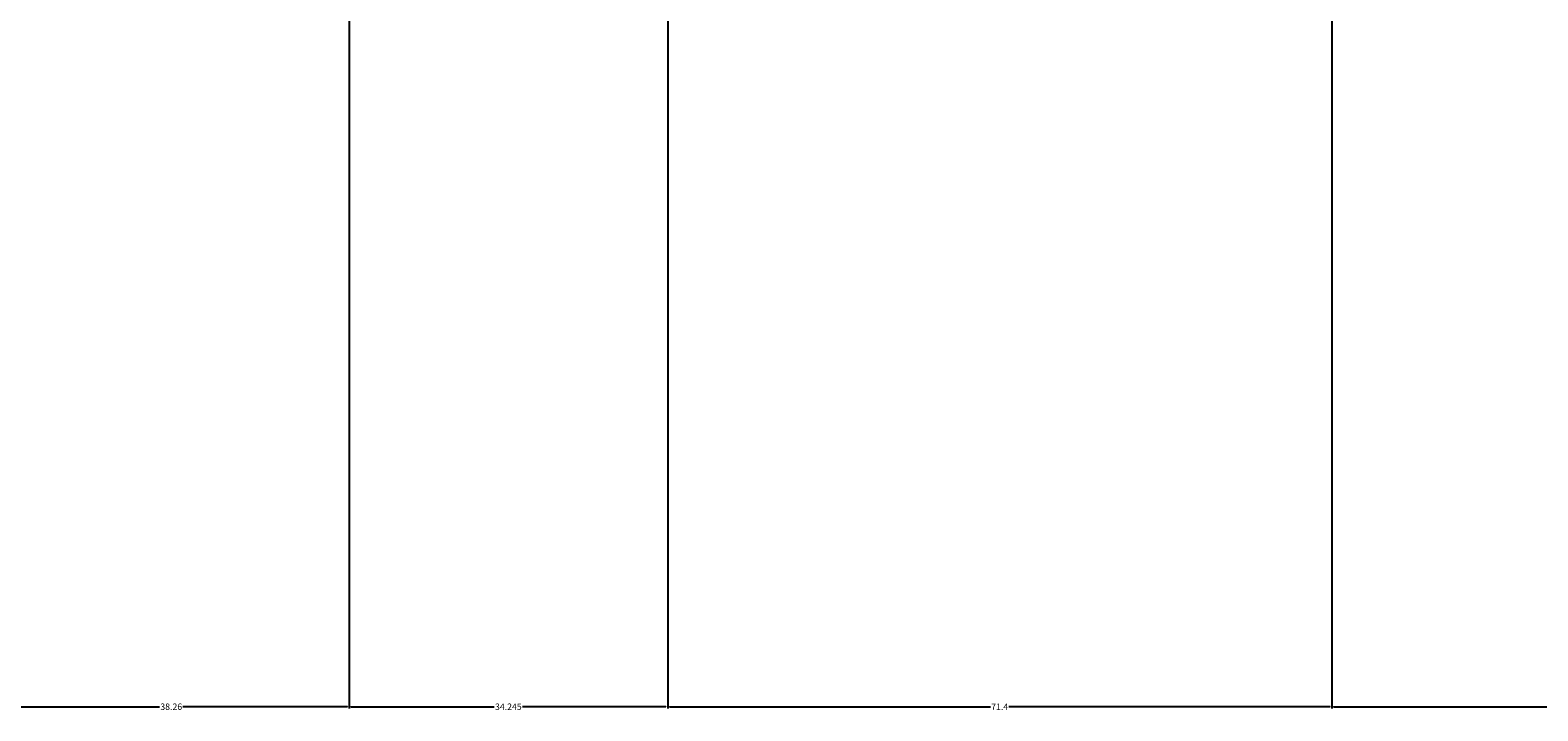
# Model space of a CAD drawing. Units: inches. Extents: x -145 to 510, y 5 to 386.
# Tile 4 of 25: x 20 to 182, y 5 to 78. Entities that reach past the tile are written whole.
import ezdxf

# ---------------------------------------------------------------- set-up
doc = ezdxf.new("R2010")
doc.units = ezdxf.units.IN
doc.header["$MEASUREMENT"] = 0
doc.layers.add('A-ANNO-DIMS', color=2, linetype='Continuous', lineweight=18)
doc.styles.get("Standard").update_dxf_attribs({"font": 'arial.ttf'})
doc.dimstyles.get("Standard").update_dxf_attribs({"dimtxt": 0.6875, "dimasz": 0.18, "dimexe": 0.18, "dimexo": 0.0625, "dimgap": 0.09, "dimtad": 0, "dimtih": 1, "dimtoh": 1, "dimdec": 4, "dimzin": 0, "dimdsep": 46, "dimlunit": 4, "dimtxsty": 'Standard', "dimcen": 0.09, "dimadec": 0, "dimazin": 0, "dimtfac": 1, "dimtdec": 4, "dimtofl": 0, "dimtmove": 0, "dimatfit": 3, "dimfxl": 1, "dimtolj": 1, "dimtzin": 0, "dimarcsym": 0})

# ---------------------------------------------------------------- blocks, each defined once
blk = doc.blocks.new('*D7')
at = {"layer": 'A-ANNO-DIMS', "color": 0, "lineweight": -2, "transparency": 16777216}
for p, q in [((88.25, 115.23), (88.25, 5.19)), ((54, 79.83), (54, 5.19)), ((54.18, 5.37), (69.6, 5.37)), ((88.07, 5.37), (72.64, 5.37))]:
    blk.add_line(p, q, dxfattribs=at)
at = {"layer": 'A-ANNO-DIMS', "color": 0, "transparency": 16777216}
for points in [[(54.18, 5.4), (54.18, 5.34), (54, 5.37)], [(88.07, 5.4), (88.07, 5.34), (88.25, 5.37)]]:
    blk.add_solid(points, dxfattribs=at)
at = {"layer": 'Defpoints', "color": 0, "transparency": 16777216}
for p in [(88.25, 115.29), (54, 79.89), (88.25, 5.37)]:
    blk.add_point(p, dxfattribs=at)
at = {"layer": 'A-ANNO-DIMS', "color": 0, "transparency": 16777216, "insert": (71.12, 5.37), "char_height": 0.688, "attachment_point": 5}
blk.add_mtext('\\A1;34.245', dxfattribs=at)
blk = doc.blocks.new('*D8')
at = {"layer": 'A-ANNO-DIMS', "color": 0, "lineweight": -2, "transparency": 16777216}
for p, q in [((88.25, 115.23), (88.25, 5.19)), ((159.65, 115.23), (159.65, 5.19)), ((88.43, 5.37), (122.97, 5.37)), ((159.47, 5.37), (124.93, 5.37))]:
    blk.add_line(p, q, dxfattribs=at)
at = {"layer": 'A-ANNO-DIMS', "color": 0, "transparency": 16777216}
for points in [[(88.43, 5.4), (88.43, 5.34), (88.25, 5.37)], [(159.47, 5.4), (159.47, 5.34), (159.65, 5.37)]]:
    blk.add_solid(points, dxfattribs=at)
at = {"layer": 'Defpoints', "color": 0, "transparency": 16777216}
for p in [(88.25, 115.29), (159.65, 115.29), (159.65, 5.37)]:
    blk.add_point(p, dxfattribs=at)
at = {"layer": 'A-ANNO-DIMS', "color": 0, "transparency": 16777216, "insert": (123.95, 5.37), "char_height": 0.688, "attachment_point": 5}
blk.add_mtext('\\A1;71.4', dxfattribs=at)
blk = doc.blocks.new('*D9')
at = {"layer": 'A-ANNO-DIMS', "color": 0, "lineweight": -2, "transparency": 16777216}
for p, q in [((159.65, 115.23), (159.65, 5.19)), ((221.53, 85.2), (221.53, 5.19)), ((159.83, 5.37), (189.34, 5.37)), ((221.35, 5.37), (191.84, 5.37))]:
    blk.add_line(p, q, dxfattribs=at)
at = {"layer": 'A-ANNO-DIMS', "color": 0, "transparency": 16777216}
for points in [[(159.83, 5.4), (159.83, 5.34), (159.65, 5.37)], [(221.35, 5.4), (221.35, 5.34), (221.53, 5.37)]]:
    blk.add_solid(points, dxfattribs=at)
at = {"layer": 'Defpoints', "color": 0, "transparency": 16777216}
for p in [(159.65, 115.29), (221.53, 85.26), (221.53, 5.37)]:
    blk.add_point(p, dxfattribs=at)
at = {"layer": 'A-ANNO-DIMS', "color": 0, "transparency": 16777216, "insert": (190.59, 5.37), "char_height": 0.688, "attachment_point": 5}
blk.add_mtext('\\A1;61.88', dxfattribs=at)
blk = doc.blocks.new('*D41')
at = {"layer": 'A-ANNO-DIMS', "color": 0, "lineweight": -2, "transparency": 16777216}
for p, q in [((15.74, 109.06), (15.74, 5.19)), ((54, 79.83), (54, 5.19)), ((15.92, 5.37), (33.62, 5.37)), ((53.82, 5.37), (36.12, 5.37))]:
    blk.add_line(p, q, dxfattribs=at)
at = {"layer": 'A-ANNO-DIMS', "color": 0, "transparency": 16777216}
for points in [[(15.92, 5.4), (15.92, 5.34), (15.74, 5.37)], [(53.82, 5.4), (53.82, 5.34), (54, 5.37)]]:
    blk.add_solid(points, dxfattribs=at)
at = {"layer": 'Defpoints', "color": 0, "transparency": 16777216}
for p in [(15.74, 109.12), (54, 79.89), (54, 5.37)]:
    blk.add_point(p, dxfattribs=at)
at = {"layer": 'A-ANNO-DIMS', "color": 0, "transparency": 16777216, "insert": (34.87, 5.37), "char_height": 0.688, "attachment_point": 5}
blk.add_mtext('\\A1;38.26', dxfattribs=at)

msp = doc.modelspace()

# ---------------------------------------------------------------- dimensions: what is measured, and where the dimension line sits
at = {"layer": 'A-ANNO-DIMS'}
for base, p1, p2, override, picture, middle in [((88.2462, 5.3738), (54.0014, 79.8905), (88.2462, 115.2922), {"dimdec": 3, "dimlfac": 1, "dimrnd": 0, "dimzin": 0, "dimdsep": 46, "dimlunit": 2}, '*D7', (71.1238, 5.3738)), ((159.6492, 5.3738), (88.2462, 115.2922), (159.6492, 115.2922), {"dimdec": 1, "dimlfac": 1, "dimrnd": 0, "dimzin": 0, "dimdsep": 46, "dimlunit": 2}, '*D8', (123.9477, 5.3738)), ((221.5292, 5.3738), (159.6492, 115.2922), (221.5292, 85.2638), {"dimdec": 2, "dimlfac": 1, "dimrnd": 0, "dimzin": 0, "dimdsep": 46, "dimlunit": 2}, '*D9', (190.5892, 5.3738)), ((54.0014, 5.3738), (15.7444, 109.1183), (54.0014, 79.8905), {"dimdec": 2, "dimlfac": 1, "dimrnd": 0, "dimzin": 0, "dimdsep": 46, "dimlunit": 2}, '*D41', (34.8729, 5.3738))]:
    dim = msp.add_linear_dim(base=base, p1=p1, p2=p2, dimstyle='Standard', override=override, dxfattribs=at)
    dim.commit()
    dim.dimension.update_dxf_attribs({"geometry": picture, "text_midpoint": middle})

doc.saveas('drawing.dxf')
